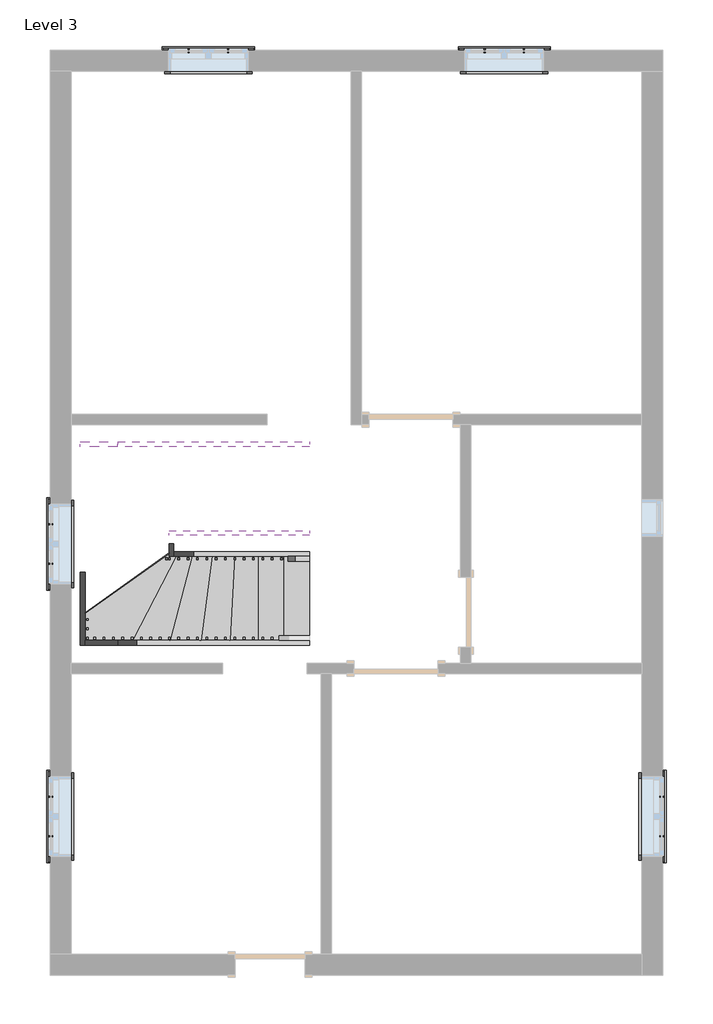
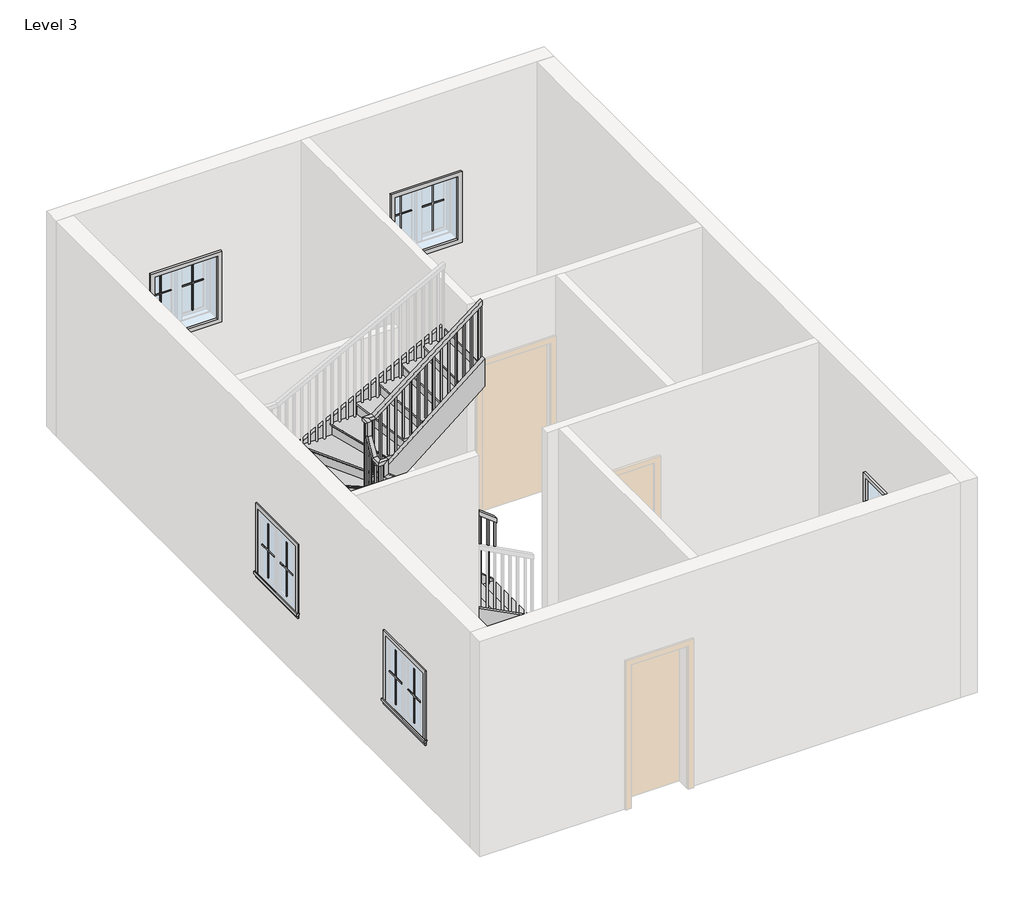
# One storey, part 2 of 2: 20 proxies, 8 members, 1 railing, 1 stair flight.
"""IFC4 building model written with IfcOpenShell, lengths in millimetres."""

from ifc_helpers import new_model, si_unit, frame, origin, place, context, project, spatial, polyline, outline, extrude, faceted_brep, transform, mapped, element, save
from components import muntin_pattern_2x2_muntin_pattern_2x2_b3fe6957, muntin_pattern_2x2_muntin_pattern_2x2_3e0ecaf2, trim_window_exterior_flat_with_sill_41619996, trim_window_interior_flat_picture_frame_51c85655, stair_flight_e257120f

model = new_model("IFC4")

# Units and contexts
model_context = context("Model", 3, world=origin())
ifc_project = project(units=[si_unit("LENGTHUNIT", "METRE", prefix="MILLI")], contexts=[model_context])

# Site, building, storey
site = spatial("IfcSite", under=ifc_project)
building = spatial("IfcBuilding", under=site)
storey = spatial("IfcBuildingStorey", under=building, Name="Level 3", Elevation=3200.4)

# Proxies
placement = place(None, origin())
muntin_pattern_2x2_muntin_pattern_2x2_shape = muntin_pattern_2x2_muntin_pattern_2x2_b3fe6957(model_context)
element("IfcBuildingElementProxy", 1, Name="Muntin Pattern_2x2 : Muntin Pattern_2x2", ObjectType="Muntin Pattern_2x2 : Muntin Pattern_2x2", at=placement, inside=storey, context=model_context, shape_type="MappedRepresentation", body=[
    mapped(muntin_pattern_2x2_muntin_pattern_2x2_shape, transform((-3096.8324167, 5150.2179147, 4184.65), x_axis=(1.0, 0.0, 0.0), y_axis=(0.0, 1.0, 0.0), z_axis=(0.0, 0.0, 1.0))),
])
element("IfcBuildingElementProxy", 2, Name="Muntin Pattern_2x2 : Muntin Pattern_2x2", ObjectType="Muntin Pattern_2x2 : Muntin Pattern_2x2", at=placement, inside=storey, context=model_context, shape_type="MappedRepresentation", body=[
    mapped(muntin_pattern_2x2_muntin_pattern_2x2_shape, transform((122.6175833, 5150.2179147, 4184.65), x_axis=(1.0, 0.0, 0.0), y_axis=(0.0, 1.0, 0.0), z_axis=(0.0, 0.0, 1.0))),
])
element("IfcBuildingElementProxy", 3, Name="Muntin Pattern_2x2 : Muntin Pattern_2x2", ObjectType="Muntin Pattern_2x2 : Muntin Pattern_2x2", at=placement, inside=storey, context=model_context, shape_type="MappedRepresentation", body=[
    mapped(muntin_pattern_2x2_muntin_pattern_2x2_shape, transform((2051.4300833, -2960.3195853, 4184.65), x_axis=(0.0, -1.0, 0.0), y_axis=(1.0, 0.0, 0.0), z_axis=(0.0, 0.0, 1.0))),
])
element("IfcBuildingElementProxy", 4, Name="Muntin Pattern_2x2 : Muntin Pattern_2x2", ObjectType="Muntin Pattern_2x2 : Muntin Pattern_2x2", at=placement, inside=storey, context=model_context, shape_type="MappedRepresentation", body=[
    mapped(muntin_pattern_2x2_muntin_pattern_2x2_shape, transform((-4597.0199167, -3388.9445853, 4184.65), x_axis=(0.0, 1.0, 0.0), y_axis=(-1.0, 0.0, 0.0), z_axis=(0.0, 0.0, 1.0))),
])
element("IfcBuildingElementProxy", 5, Name="Muntin Pattern_2x2 : Muntin Pattern_2x2", ObjectType="Muntin Pattern_2x2 : Muntin Pattern_2x2", at=placement, inside=storey, context=model_context, shape_type="MappedRepresentation", body=[
    mapped(muntin_pattern_2x2_muntin_pattern_2x2_shape, transform((-4597.0199167, -426.6695853, 4184.65), x_axis=(0.0, 1.0, 0.0), y_axis=(-1.0, 0.0, 0.0), z_axis=(0.0, 0.0, 1.0))),
])
muntin_pattern_2x2_muntin_pattern_2x2_2_shape = muntin_pattern_2x2_muntin_pattern_2x2_3e0ecaf2(model_context)
element("IfcBuildingElementProxy", 6, Name="Muntin Pattern_2x2 : Muntin Pattern_2x2", ObjectType="Muntin Pattern_2x2 : Muntin Pattern_2x2", at=placement, inside=storey, context=model_context, shape_type="MappedRepresentation", body=[
    mapped(muntin_pattern_2x2_muntin_pattern_2x2_2_shape, transform((-2668.2074167, 5150.2179147, 4184.65), x_axis=(-1.0, 0.0, 0.0), y_axis=(0.0, -1.0, 0.0), z_axis=(0.0, 0.0, 1.0))),
])
element("IfcBuildingElementProxy", 7, Name="Muntin Pattern_2x2 : Muntin Pattern_2x2", ObjectType="Muntin Pattern_2x2 : Muntin Pattern_2x2", at=placement, inside=storey, context=model_context, shape_type="MappedRepresentation", body=[
    mapped(muntin_pattern_2x2_muntin_pattern_2x2_2_shape, transform((551.2425833, 5150.2179147, 4184.65), x_axis=(-1.0, 0.0, 0.0), y_axis=(0.0, -1.0, 0.0), z_axis=(0.0, 0.0, 1.0))),
])
element("IfcBuildingElementProxy", 8, Name="Muntin Pattern_2x2 : Muntin Pattern_2x2", ObjectType="Muntin Pattern_2x2 : Muntin Pattern_2x2", at=placement, inside=storey, context=model_context, shape_type="MappedRepresentation", body=[
    mapped(muntin_pattern_2x2_muntin_pattern_2x2_2_shape, transform((2051.4300833, -3388.9445853, 4184.65), x_axis=(0.0, 1.0, 0.0), y_axis=(-1.0, 0.0, 0.0), z_axis=(0.0, 0.0, 1.0))),
])
element("IfcBuildingElementProxy", 9, Name="Muntin Pattern_2x2 : Muntin Pattern_2x2", ObjectType="Muntin Pattern_2x2 : Muntin Pattern_2x2", at=placement, inside=storey, context=model_context, shape_type="MappedRepresentation", body=[
    mapped(muntin_pattern_2x2_muntin_pattern_2x2_2_shape, transform((-4597.0199167, -2960.3195853, 4184.65), x_axis=(0.0, -1.0, 0.0), y_axis=(1.0, 0.0, 0.0), z_axis=(0.0, 0.0, 1.0))),
])
element("IfcBuildingElementProxy", 10, Name="Muntin Pattern_2x2 : Muntin Pattern_2x2", ObjectType="Muntin Pattern_2x2 : Muntin Pattern_2x2", at=placement, inside=storey, context=model_context, shape_type="MappedRepresentation", body=[
    mapped(muntin_pattern_2x2_muntin_pattern_2x2_2_shape, transform((-4597.0199167, 1.9554147, 4184.65), x_axis=(0.0, -1.0, 0.0), y_axis=(1.0, 0.0, 0.0), z_axis=(0.0, 0.0, 1.0))),
])
trim_window_exterior_flat_with_sill_shape = trim_window_exterior_flat_with_sill_41619996(model_context)
element("IfcBuildingElementProxy", 11, Name="Trim-Window-Exterior-Flat : with Sill", ObjectType="Trim-Window-Exterior-Flat : with Sill", at=placement, inside=storey, context=model_context, shape_type="MappedRepresentation", body=[
    mapped(trim_window_exterior_flat_with_sill_shape, transform((-2882.5199167, 5159.7429147, 5029.2), x_axis=(-1.0, 0.0, 0.0), y_axis=(0.0, 0.0, 1.0), z_axis=(0.0, 1.0, 0.0))),
])
element("IfcBuildingElementProxy", 12, Name="Trim-Window-Exterior-Flat : with Sill", ObjectType="Trim-Window-Exterior-Flat : with Sill", at=placement, inside=storey, context=model_context, shape_type="MappedRepresentation", body=[
    mapped(trim_window_exterior_flat_with_sill_shape, transform((336.9300833, 5159.7429147, 5029.2), x_axis=(-1.0, 0.0, 0.0), y_axis=(0.0, 0.0, 1.0), z_axis=(0.0, 1.0, 0.0))),
])
element("IfcBuildingElementProxy", 13, Name="Trim-Window-Exterior-Flat : with Sill", ObjectType="Trim-Window-Exterior-Flat : with Sill", at=placement, inside=storey, context=model_context, shape_type="MappedRepresentation", body=[
    mapped(trim_window_exterior_flat_with_sill_shape, transform((2060.9550833, -3174.6320853, 5029.2), x_axis=(0.0, 1.0, 0.0), y_axis=(0.0, 0.0, 1.0), z_axis=(1.0, 0.0, 0.0))),
])
element("IfcBuildingElementProxy", 14, Name="Trim-Window-Exterior-Flat : with Sill", ObjectType="Trim-Window-Exterior-Flat : with Sill", at=placement, inside=storey, context=model_context, shape_type="MappedRepresentation", body=[
    mapped(trim_window_exterior_flat_with_sill_shape, transform((-4606.5449167, -3174.6320853, 5029.2), x_axis=(0.0, -1.0, 0.0), y_axis=(0.0, 0.0, 1.0), z_axis=(-1.0, 0.0, 0.0))),
])
element("IfcBuildingElementProxy", 15, Name="Trim-Window-Exterior-Flat : with Sill", ObjectType="Trim-Window-Exterior-Flat : with Sill", at=placement, inside=storey, context=model_context, shape_type="MappedRepresentation", body=[
    mapped(trim_window_exterior_flat_with_sill_shape, transform((-4606.5449167, -212.3570853, 5029.2), x_axis=(0.0, -1.0, 0.0), y_axis=(0.0, 0.0, 1.0), z_axis=(-1.0, 0.0, 0.0))),
])
trim_window_interior_flat_picture_frame_shape = trim_window_interior_flat_picture_frame_51c85655(model_context)
element("IfcBuildingElementProxy", 16, Name="Trim-Window-Interior-Flat : Picture Frame", ObjectType="Trim-Window-Interior-Flat : Picture Frame", at=placement, inside=storey, context=model_context, shape_type="MappedRepresentation", body=[
    mapped(trim_window_interior_flat_picture_frame_shape, transform((-2882.5199167, 4931.1429147, 5029.2), x_axis=(1.0, 0.0, 0.0), y_axis=(0.0, 0.0, 1.0), z_axis=(0.0, -1.0, 0.0))),
])
element("IfcBuildingElementProxy", 17, Name="Trim-Window-Interior-Flat : Picture Frame", ObjectType="Trim-Window-Interior-Flat : Picture Frame", at=placement, inside=storey, context=model_context, shape_type="MappedRepresentation", body=[
    mapped(trim_window_interior_flat_picture_frame_shape, transform((336.9300833, 4931.1429147, 5029.2), x_axis=(1.0, 0.0, 0.0), y_axis=(0.0, 0.0, 1.0), z_axis=(0.0, -1.0, 0.0))),
])
element("IfcBuildingElementProxy", 18, Name="Trim-Window-Interior-Flat : Picture Frame", ObjectType="Trim-Window-Interior-Flat : Picture Frame", at=placement, inside=storey, context=model_context, shape_type="MappedRepresentation", body=[
    mapped(trim_window_interior_flat_picture_frame_shape, transform((1832.3550833, -3174.6320853, 5029.2), x_axis=(0.0, -1.0, 0.0), y_axis=(0.0, 0.0, 1.0), z_axis=(-1.0, 0.0, 0.0))),
])
element("IfcBuildingElementProxy", 19, Name="Trim-Window-Interior-Flat : Picture Frame", ObjectType="Trim-Window-Interior-Flat : Picture Frame", at=placement, inside=storey, context=model_context, shape_type="MappedRepresentation", body=[
    mapped(trim_window_interior_flat_picture_frame_shape, transform((-4377.9449167, -3174.6320853, 5029.2), x_axis=(0.0, 1.0, 0.0), y_axis=(0.0, 0.0, 1.0), z_axis=(1.0, 0.0, 0.0))),
])
element("IfcBuildingElementProxy", 20, Name="Trim-Window-Interior-Flat : Picture Frame", ObjectType="Trim-Window-Interior-Flat : Picture Frame", at=placement, inside=storey, context=model_context, shape_type="MappedRepresentation", body=[
    mapped(trim_window_interior_flat_picture_frame_shape, transform((-4377.9449167, -212.3570853, 5029.2), x_axis=(0.0, 1.0, 0.0), y_axis=(0.0, 0.0, 1.0), z_axis=(1.0, 0.0, 0.0))),
])

# Members
element("IfcMember", 21, ObjectType="Stringer - 2\" Width", at=placement, inside=storey, context=model_context, shape_type="SweptSolid", body=[
    extrude(outline(polyline([(3200.4, -1783.4132248), (3430.039954, -1783.4132248), (4505.7956453, -3870.8304165), (4162.900629, -3870.8304165), (3200.4, -2003.1755424), (3200.4, -1783.4132248)])), frame((0.0, -1310.9070853, 0.0), z_axis=(0.0, 1.0, 0.0), x_axis=(0.0, 0.0, 1.0)), (0.0, 0.0, 1.0), 50.8),
])
element("IfcMember", 22, ObjectType="Stringer - 2\" Width", at=placement, inside=storey, context=model_context, shape_type="SweptSolid", body=[
    extrude(outline(polyline([(-3870.8304165, -1260.1070853), (-3870.8304165, -1310.9070853), (-4225.5449167, -1310.9070853), (-4225.5449167, -1260.1070853), (-3870.8304165, -1260.1070853)])), frame((0.0, 0.0, 4162.900629), z_axis=(0.0, 0.0, 1.0), x_axis=(1.0, 0.0, 0.0)), (0.0, 0.0, 1.0), 342.8950162),
])
element("IfcMember", 23, ObjectType="Stringer - 2\" Width", at=placement, inside=storey, context=model_context, shape_type="SweptSolid", body=[
    extrude(outline(polyline([(-1310.9070853, 4200.9956453), (-1310.9070853, 4489.4952212), (811.1127974, 5170.3972697), (848.0929147, 5170.3972697), (848.0929147, 4839.3682298), (-1141.3846024, 4200.9956453), (-1310.9070853, 4200.9956453)])), frame((-4276.3449167, 0.0, 0.0), z_axis=(1.0, 0.0, 0.0), x_axis=(0.0, 1.0, 0.0)), (0.0, 0.0, 1.0), 50.8),
])
element("IfcMember", 24, ObjectType="Stringer - 2\" Width", at=placement, inside=storey, context=model_context, shape_type="SweptSolid", body=[
    extrude(outline(polyline([(-4276.3449167, 848.0929147), (-4276.3449167, 898.8929147), (-3870.8304165, 898.8929147), (-3870.8304165, 848.0929147), (-4276.3449167, 848.0929147)])), frame((0.0, 0.0, 4850.2904473), z_axis=(0.0, 0.0, 1.0), x_axis=(1.0, 0.0, 0.0)), (0.0, 0.0, 1.0), 320.1068224),
])
element("IfcMember", 25, ObjectType="Stringer - 2\" Width", at=placement, inside=storey, context=model_context, shape_type="SweptSolid", body=[
    extrude(outline(polyline([(5170.3972697, -3870.8304165), (4850.2904473, -3870.8304165), (5926.0461385, -1783.4132248), (6246.1529609, -1783.4132248), (5170.3972697, -3870.8304165)])), frame((0.0, 848.0929147, 0.0), z_axis=(0.0, 1.0, 0.0), x_axis=(0.0, 0.0, 1.0)), (0.0, 0.0, 1.0), 50.8),
])
element("IfcMember", 26, ObjectType="Stringer - 2\" Width", at=placement, inside=storey, context=model_context, shape_type="SweptSolid", body=[
    extrude(outline(polyline([(3200.4, -1783.4132248), (3376.5764461, -1783.4132248), (4580.818648, -3260.3449167), (4187.5410923, -3260.3449167), (3200.4, -2049.6748694), (3200.4, -1783.4132248)])), frame((0.0, -345.7070853, 0.0), z_axis=(0.0, 1.0, 0.0), x_axis=(0.0, 0.0, 1.0)), (0.0, 0.0, 1.0), 50.8),
])
element("IfcMember", 27, ObjectType="Stringer - 2\" Width", at=placement, inside=storey, context=model_context, shape_type="SweptSolid", body=[
    extrude(outline(polyline([(-345.7070853, 4228.9617647), (-345.7070853, 4773.6682978), (-139.0699679, 5126.5409689), (-117.1070853, 5126.5409689), (-117.1070853, 4560.865107), (-311.464868, 4228.9617647), (-345.7070853, 4228.9617647)])), frame((-3311.1449167, 0.0, 0.0), z_axis=(1.0, 0.0, 0.0), x_axis=(0.0, 1.0, 0.0)), (0.0, 0.0, 1.0), 50.8),
])
element("IfcMember", 28, ObjectType="Stringer - 2\" Width", at=placement, inside=storey, context=model_context, shape_type="SweptSolid", body=[
    extrude(outline(polyline([(5126.5409689, -3311.1449167), (4733.2634131, -3311.1449167), (5978.9262875, -1783.4132248), (6372.2038432, -1783.4132248), (5126.5409689, -3311.1449167)])), frame((0.0, -117.1070853, 0.0), z_axis=(0.0, 1.0, 0.0), x_axis=(0.0, 0.0, 1.0)), (0.0, 0.0, 1.0), 50.8),
])

# Railing
element("IfcRailing", 29, ObjectType="Handrail - Rectangular", at=placement, inside=storey, context=model_context, shape_type="SolidModel", body=[
    faceted_brep([(-1783.4132248, -396.5070853, 4284.1333333), (-1783.4132248, -396.5070853, 4219.8000346), (-1783.4132248, -345.7070853, 4219.8000346), (-1783.4132248, -345.7070853, 4284.1333333), (-3234.9449167, -396.5070853, 5412.0191036), (-3285.7449167, -396.5070853, 5387.1590024), (-3285.7449167, -345.7070853, 5387.1590024), (-3234.9449167, -345.7070853, 5412.0191036), (-3234.9449167, -396.5070853, 5615.0281882), (-3285.7449167, -396.5070853, 5564.2281882), (-3285.7449167, -345.7070853, 5564.2281882), (-3234.9449167, -345.7070853, 5615.0281882), (-3361.9449167, -396.5070853, 5615.0281882), (-3361.9449167, -396.5070853, 5564.2281882), (-3311.1449167, -345.7070853, 5564.2281882), (-3311.1449167, -345.7070853, 5615.0281882), (-3361.9449167, -269.5070853, 5615.0281882), (-3361.9449167, -240.3857515, 5564.2281882), (-3311.1449167, -240.3857515, 5564.2281882), (-3311.1449167, -269.5070853, 5615.0281882), (-3361.9449167, -142.5070853, 5831.9051451), (-3361.9449167, -91.7070853, 5818.1256424), (-3311.1449167, -91.7070853, 5818.1256424), (-3311.1449167, -142.5070853, 5831.9051451), (-3361.9449167, -142.5070853, 6034.9142297), (-3361.9449167, -91.7070853, 5984.1142297), (-3311.1449167, -91.7070853, 5984.1142297), (-3311.1449167, -142.5070853, 6034.9142297), (-3361.9449167, -15.5070853, 6034.9142297), (-3361.9449167, -15.5070853, 5984.1142297), (-3311.1449167, -66.3070853, 5984.1142297), (-3311.1449167, -66.3070853, 6034.9142297), (-3234.9449167, -15.5070853, 6034.9142297), (-3217.5282487, -15.5070853, 5984.1142297), (-3217.5282487, -66.3070853, 5984.1142297), (-3234.9449167, -66.3070853, 6034.9142297), (-1783.4132248, -15.5070853, 7162.8), (-1783.4132248, -66.3070853, 7162.8), (-1783.4132248, -66.3070853, 7098.4667013), (-1783.4132248, -15.5070853, 7098.4667013)], [[[0, 1, 2, 3]], [[1, 0, 4, 5]], [[2, 1, 5, 6]], [[3, 2, 6, 7]], [[0, 3, 7, 4]], [[5, 4, 8, 9]], [[6, 5, 9, 10]], [[7, 6, 10, 11]], [[4, 7, 11, 8]], [[9, 8, 12, 13]], [[10, 9, 13, 14]], [[11, 10, 14, 15]], [[8, 11, 15, 12]], [[13, 12, 16, 17]], [[14, 13, 17, 18]], [[15, 14, 18, 19]], [[12, 15, 19, 16]], [[17, 16, 20, 21]], [[18, 17, 21, 22]], [[19, 18, 22, 23]], [[16, 19, 23, 20]], [[21, 20, 24, 25]], [[22, 21, 25, 26]], [[23, 22, 26, 27]], [[20, 23, 27, 24]], [[25, 24, 28, 29]], [[26, 25, 29, 30]], [[27, 26, 30, 31]], [[24, 27, 31, 28]], [[29, 28, 32, 33]], [[30, 29, 33, 34]], [[31, 30, 34, 35]], [[28, 31, 35, 32]], [[36, 37, 38, 39]], [[33, 32, 36, 39]], [[34, 33, 39, 38]], [[35, 34, 38, 37]], [[32, 35, 37, 36]]]),
    extrude(outline(polyline([(7083.2316852, -1803.0199167), (7068.4292361, -1822.0699167), (6079.0666667, -1822.0699167), (6079.0666667, -1803.0199167), (7083.2316852, -1803.0199167)])), frame((0.0, -50.4320853, 0.0), z_axis=(0.0, 1.0, 0.0), x_axis=(0.0, 0.0, 1.0)), (0.0, 0.0, 1.0), 19.05),
    extrude(outline(polyline([(7004.2852902, -1904.6199167), (6989.4828411, -1923.6699167), (6079.0666667, -1923.6699167), (6079.0666667, -1904.6199167), (7004.2852902, -1904.6199167)])), frame((0.0, -50.4320853, 0.0), z_axis=(0.0, 1.0, 0.0), x_axis=(0.0, 0.0, 1.0)), (0.0, 0.0, 1.0), 19.05),
    extrude(outline(polyline([(6925.3388952, -2006.2199167), (6910.5364462, -2025.2699167), (6079.0666667, -2025.2699167), (6079.0666667, -2006.2199167), (6925.3388952, -2006.2199167)])), frame((0.0, -50.4320853, 0.0), z_axis=(0.0, 1.0, 0.0), x_axis=(0.0, 0.0, 1.0)), (0.0, 0.0, 1.0), 19.05),
    extrude(outline(polyline([(6846.3925003, -2107.8199167), (6831.5900512, -2126.8699167), (5909.7333333, -2126.8699167), (5909.7333333, -2107.8199167), (6846.3925003, -2107.8199167)])), frame((0.0, -50.4320853, 0.0), z_axis=(0.0, 1.0, 0.0), x_axis=(0.0, 0.0, 1.0)), (0.0, 0.0, 1.0), 19.05),
    extrude(outline(polyline([(6767.4461053, -2209.4199167), (6752.6436562, -2228.4699167), (5909.7333333, -2228.4699167), (5909.7333333, -2209.4199167), (6767.4461053, -2209.4199167)])), frame((0.0, -50.4320853, 0.0), z_axis=(0.0, 1.0, 0.0), x_axis=(0.0, 0.0, 1.0)), (0.0, 0.0, 1.0), 19.05),
    extrude(outline(polyline([(6688.4997103, -2311.0199167), (6673.6972613, -2330.0699167), (5909.7333333, -2330.0699167), (5909.7333333, -2311.0199167), (6688.4997103, -2311.0199167)])), frame((0.0, -50.4320853, 0.0), z_axis=(0.0, 1.0, 0.0), x_axis=(0.0, 0.0, 1.0)), (0.0, 0.0, 1.0), 19.05),
    extrude(outline(polyline([(6609.5533154, -2412.6199167), (6594.7508663, -2431.6699167), (5740.4, -2431.6699167), (5740.4, -2412.6199167), (6609.5533154, -2412.6199167)])), frame((0.0, -50.4320853, 0.0), z_axis=(0.0, 1.0, 0.0), x_axis=(0.0, 0.0, 1.0)), (0.0, 0.0, 1.0), 19.05),
    extrude(outline(polyline([(6530.6069204, -2514.2199167), (6515.8044713, -2533.2699167), (5740.4, -2533.2699167), (5740.4, -2514.2199167), (6530.6069204, -2514.2199167)])), frame((0.0, -50.4320853, 0.0), z_axis=(0.0, 1.0, 0.0), x_axis=(0.0, 0.0, 1.0)), (0.0, 0.0, 1.0), 19.05),
    extrude(outline(polyline([(6451.6605254, -2615.8199167), (6436.8580764, -2634.8699167), (5571.0666667, -2634.8699167), (5571.0666667, -2615.8199167), (6451.6605254, -2615.8199167)])), frame((0.0, -50.4320853, 0.0), z_axis=(0.0, 1.0, 0.0), x_axis=(0.0, 0.0, 1.0)), (0.0, 0.0, 1.0), 19.05),
    extrude(outline(polyline([(6372.7141304, -2717.4199167), (6357.9116814, -2736.4699167), (5571.0666667, -2736.4699167), (5571.0666667, -2717.4199167), (6372.7141304, -2717.4199167)])), frame((0.0, -50.4320853, 0.0), z_axis=(0.0, 1.0, 0.0), x_axis=(0.0, 0.0, 1.0)), (0.0, 0.0, 1.0), 19.05),
    extrude(outline(polyline([(6293.7677355, -2819.0199167), (6278.9652864, -2838.0699167), (5571.0666667, -2838.0699167), (5571.0666667, -2819.0199167), (6293.7677355, -2819.0199167)])), frame((0.0, -50.4320853, 0.0), z_axis=(0.0, 1.0, 0.0), x_axis=(0.0, 0.0, 1.0)), (0.0, 0.0, 1.0), 19.05),
    extrude(outline(polyline([(6214.8213405, -2920.6199167), (6200.0188914, -2939.6699167), (5401.7333333, -2939.6699167), (5401.7333333, -2920.6199167), (6214.8213405, -2920.6199167)])), frame((0.0, -50.4320853, 0.0), z_axis=(0.0, 1.0, 0.0), x_axis=(0.0, 0.0, 1.0)), (0.0, 0.0, 1.0), 19.05),
    extrude(outline(polyline([(6135.8749455, -3022.2199167), (6121.0724965, -3041.2699167), (5401.7333333, -3041.2699167), (5401.7333333, -3022.2199167), (6135.8749455, -3022.2199167)])), frame((0.0, -50.4320853, 0.0), z_axis=(0.0, 1.0, 0.0), x_axis=(0.0, 0.0, 1.0)), (0.0, 0.0, 1.0), 19.05),
    extrude(outline(polyline([(6056.9285506, -3123.8199167), (6042.1261015, -3142.8699167), (5232.4, -3142.8699167), (5232.4, -3123.8199167), (6056.9285506, -3123.8199167)])), frame((0.0, -50.4320853, 0.0), z_axis=(0.0, 1.0, 0.0), x_axis=(0.0, 0.0, 1.0)), (0.0, 0.0, 1.0), 19.05),
    extrude(outline(polyline([(5977.9821556, -3225.4199167), (5963.1797065, -3244.4699167), (5232.4, -3244.4699167), (5232.4, -3225.4199167), (5977.9821556, -3225.4199167)])), frame((0.0, -50.4320853, 0.0), z_axis=(0.0, 1.0, 0.0), x_axis=(0.0, 0.0, 1.0)), (0.0, 0.0, 1.0), 19.05),
    extrude(outline(polyline([(-3327.0199167, -75.8320853), (-3346.0699167, -75.8320853), (-3346.0699167, -56.7820853), (-3327.0199167, -56.7820853), (-3327.0199167, -75.8320853)])), frame((0.0, 0.0, 4893.7333333), z_axis=(0.0, 0.0, 1.0), x_axis=(1.0, 0.0, 0.0)), (0.0, 0.0, 1.0), 1090.3808964),
    extrude(outline(polyline([(-177.4320853, 5671.7336964), (-158.3820853, 5704.26524), (-158.3820853, 4724.4), (-177.4320853, 4724.4), (-177.4320853, 5671.7336964)])), frame((-3346.0699167, 0.0, 0.0), z_axis=(1.0, 0.0, 0.0), x_axis=(0.0, 1.0, 0.0)), (0.0, 0.0, 1.0), 19.05),
    extrude(outline(polyline([(-279.0320853, 5498.2321309), (-259.9820853, 5530.7636744), (-259.9820853, 4555.0666667), (-279.0320853, 4555.0666667), (-279.0320853, 5498.2321309)])), frame((-3346.0699167, 0.0, 0.0), z_axis=(1.0, 0.0, 0.0), x_axis=(0.0, 1.0, 0.0)), (0.0, 0.0, 1.0), 19.05),
    extrude(outline(polyline([(-3297.8882248, -361.5820853), (-3297.8882248, -380.6320853), (-3316.9382248, -380.6320853), (-3316.9382248, -361.5820853), (-3297.8882248, -361.5820853)])), frame((0.0, 0.0, 4385.7333333), z_axis=(0.0, 0.0, 1.0), x_axis=(1.0, 0.0, 0.0)), (0.0, 0.0, 1.0), 1178.4948549),
    extrude(outline(polyline([(5317.6483397, -3196.2882248), (5332.4507888, -3215.3382248), (4216.4, -3215.3382248), (4216.4, -3196.2882248), (5317.6483397, -3196.2882248)])), frame((0.0, -380.6320853, 0.0), z_axis=(0.0, 1.0, 0.0), x_axis=(0.0, 0.0, 1.0)), (0.0, 0.0, 1.0), 19.05),
    extrude(outline(polyline([(5238.7019447, -3094.6882248), (5253.5043938, -3113.7382248), (4216.4, -3113.7382248), (4216.4, -3094.6882248), (5238.7019447, -3094.6882248)])), frame((0.0, -380.6320853, 0.0), z_axis=(0.0, 1.0, 0.0), x_axis=(0.0, 0.0, 1.0)), (0.0, 0.0, 1.0), 19.05),
    extrude(outline(polyline([(5159.7555498, -2993.0882248), (5174.5579988, -3012.1382248), (4047.0666667, -3012.1382248), (4047.0666667, -2993.0882248), (5159.7555498, -2993.0882248)])), frame((0.0, -380.6320853, 0.0), z_axis=(0.0, 1.0, 0.0), x_axis=(0.0, 0.0, 1.0)), (0.0, 0.0, 1.0), 19.05),
    extrude(outline(polyline([(5080.8091548, -2891.4882248), (5095.6116039, -2910.5382248), (4047.0666667, -2910.5382248), (4047.0666667, -2891.4882248), (5080.8091548, -2891.4882248)])), frame((0.0, -380.6320853, 0.0), z_axis=(0.0, 1.0, 0.0), x_axis=(0.0, 0.0, 1.0)), (0.0, 0.0, 1.0), 19.05),
    extrude(outline(polyline([(5001.8627598, -2789.8882248), (5016.6652089, -2808.9382248), (3877.7333333, -2808.9382248), (3877.7333333, -2789.8882248), (5001.8627598, -2789.8882248)])), frame((0.0, -380.6320853, 0.0), z_axis=(0.0, 1.0, 0.0), x_axis=(0.0, 0.0, 1.0)), (0.0, 0.0, 1.0), 19.05),
    extrude(outline(polyline([(4922.9163649, -2688.2882248), (4937.7188139, -2707.3382248), (3877.7333333, -2707.3382248), (3877.7333333, -2688.2882248), (4922.9163649, -2688.2882248)])), frame((0.0, -380.6320853, 0.0), z_axis=(0.0, 1.0, 0.0), x_axis=(0.0, 0.0, 1.0)), (0.0, 0.0, 1.0), 19.05),
    extrude(outline(polyline([(4843.9699699, -2586.6882248), (4858.7724189, -2605.7382248), (3708.4, -2605.7382248), (3708.4, -2586.6882248), (4843.9699699, -2586.6882248)])), frame((0.0, -380.6320853, 0.0), z_axis=(0.0, 1.0, 0.0), x_axis=(0.0, 0.0, 1.0)), (0.0, 0.0, 1.0), 19.05),
    extrude(outline(polyline([(4765.0235749, -2485.0882248), (4779.826024, -2504.1382248), (3708.4, -2504.1382248), (3708.4, -2485.0882248), (4765.0235749, -2485.0882248)])), frame((0.0, -380.6320853, 0.0), z_axis=(0.0, 1.0, 0.0), x_axis=(0.0, 0.0, 1.0)), (0.0, 0.0, 1.0), 19.05),
    extrude(outline(polyline([(4686.0771799, -2383.4882248), (4700.879629, -2402.5382248), (3708.4, -2402.5382248), (3708.4, -2383.4882248), (4686.0771799, -2383.4882248)])), frame((0.0, -380.6320853, 0.0), z_axis=(0.0, 1.0, 0.0), x_axis=(0.0, 0.0, 1.0)), (0.0, 0.0, 1.0), 19.05),
    extrude(outline(polyline([(4607.130785, -2281.8882248), (4621.933234, -2300.9382248), (3539.0666667, -2300.9382248), (3539.0666667, -2281.8882248), (4607.130785, -2281.8882248)])), frame((0.0, -380.6320853, 0.0), z_axis=(0.0, 1.0, 0.0), x_axis=(0.0, 0.0, 1.0)), (0.0, 0.0, 1.0), 19.05),
    extrude(outline(polyline([(4528.18439, -2180.2882248), (4542.9868391, -2199.3382248), (3539.0666667, -2199.3382248), (3539.0666667, -2180.2882248), (4528.18439, -2180.2882248)])), frame((0.0, -380.6320853, 0.0), z_axis=(0.0, 1.0, 0.0), x_axis=(0.0, 0.0, 1.0)), (0.0, 0.0, 1.0), 19.05),
    extrude(outline(polyline([(4449.237995, -2078.6882248), (4464.0404441, -2097.7382248), (3539.0666667, -2097.7382248), (3539.0666667, -2078.6882248), (4449.237995, -2078.6882248)])), frame((0.0, -380.6320853, 0.0), z_axis=(0.0, 1.0, 0.0), x_axis=(0.0, 0.0, 1.0)), (0.0, 0.0, 1.0), 19.05),
    extrude(outline(polyline([(4370.2916001, -1977.0882248), (4385.0940491, -1996.1382248), (3369.7333333, -1996.1382248), (3369.7333333, -1977.0882248), (4370.2916001, -1977.0882248)])), frame((0.0, -380.6320853, 0.0), z_axis=(0.0, 1.0, 0.0), x_axis=(0.0, 0.0, 1.0)), (0.0, 0.0, 1.0), 19.05),
    extrude(outline(polyline([(4291.3452051, -1875.4882248), (4306.1476541, -1894.5382248), (3369.7333333, -1894.5382248), (3369.7333333, -1875.4882248), (4291.3452051, -1875.4882248)])), frame((0.0, -380.6320853, 0.0), z_axis=(0.0, 1.0, 0.0), x_axis=(0.0, 0.0, 1.0)), (0.0, 0.0, 1.0), 19.05),
    extrude(outline(polyline([(-3327.0199167, -50.4320853), (-3346.0699167, -50.4320853), (-3346.0699167, -31.3820853), (-3327.0199167, -31.3820853), (-3327.0199167, -50.4320853)])), frame((0.0, 0.0, 5063.0666667), z_axis=(0.0, 0.0, 1.0), x_axis=(1.0, 0.0, 0.0)), (0.0, 0.0, 1.0), 921.0475631),
    extrude(outline(polyline([(-3327.0199167, -361.5820853), (-3327.0199167, -380.6320853), (-3346.0699167, -380.6320853), (-3346.0699167, -361.5820853), (-3327.0199167, -361.5820853)])), frame((0.0, 0.0, 4385.7333333), z_axis=(0.0, 0.0, 1.0), x_axis=(1.0, 0.0, 0.0)), (0.0, 0.0, 1.0), 1178.4948549),
    extrude(outline(polyline([(7098.4667013, -1783.4132248), (7083.6642523, -1802.4632248), (6079.0666667, -1802.4632248), (6079.0666667, -1783.4132248), (7098.4667013, -1783.4132248)])), frame((0.0, -50.4320853, 0.0), z_axis=(0.0, 1.0, 0.0), x_axis=(0.0, 0.0, 1.0)), (0.0, 0.0, 1.0), 19.05),
    extrude(outline(polyline([(4219.8000346, -1783.4132248), (4234.6024837, -1802.4632248), (3369.7333333, -1802.4632248), (3369.7333333, -1783.4132248), (4219.8000346, -1783.4132248)])), frame((0.0, -380.6320853, 0.0), z_axis=(0.0, 1.0, 0.0), x_axis=(0.0, 0.0, 1.0)), (0.0, 0.0, 1.0), 19.05),
])

# Stair flight
stair_flight_shape = stair_flight_e257120f(model_context)
element("IfcStairFlight", 30, ObjectType="2\" Tread 1\" Nosing 1/4\" Riser", at=placement, inside=storey, context=model_context, shape_type="MappedRepresentation", body=[
    mapped(stair_flight_shape, transform((0.0, 0.0, 0.0), x_axis=(1.0, 0.0, 0.0), y_axis=(0.0, 1.0, 0.0), z_axis=(0.0, 0.0, 1.0))),
])

save(model, "model.ifc")

# Revit data of these elements
# Type "Muntin Pattern_2x2 : Muntin Pattern_2x2"
#   Width [instance default] = 4' - 0"
#   Thickness = 0' - 0 1/2"
#   Height [instance default] = 4' - 0"
#   Distance = 0' - 0 3/4"
#   Interior Material [instance default] = none
#   Exterior Material [instance default] = none
#   Default Elevation = 0
# Type "Trim-Window-Exterior-Flat : with Sill"
#   Trim Width = 0' - 2 1/4"
#   Trim Thickness_Picture Frame = 0' - 1 1/4"
#   Trim Thickness_with Sill = 0' - 0 3/4"
#   Sill Thickness = 0' - 1 1/4"
#   Opening Width [instance default] = 2' - 0"
#   Opening Height [instance default] = 3' - 0"
#   Default Elevation = 4' - 0"
#   Sill = yes
#   Picture Frame = no
#   Trim Material [instance default] = none
# Type "Trim-Window-Interior-Flat : Picture Frame"
#   Trim Thickness_Picture Frame = 0' - 1 1/4"
#   Trim Width = 0' - 2 1/4"
#   Trim Thickness_with Sill = 0' - 0 3/4"
#   Sill Thickness = 0' - 1 1/4"
#   Opening Width [instance default] = 2' - 0"
#   Opening Height [instance default] = 3' - 0"
#   Default Elevation = 4' - 0"
#   Sill = no
#   Picture Frame = yes
#   Trim Material [instance default] = none
# Type "Handrail - Rectangular"
#   Assembly Code = "C2010400"
#   built-in parameter 1008612 = 0.0416667 (stored number, unit not read)
#   built-in parameter 1008611 = 0.0416667 (stored number, unit not read)
#   built-in parameter 1008609 = 0.333333 (stored number, unit not read)
#   built-in parameter 1008604 = 0.166667 (stored number, unit not read)
#   built-in parameter 1008603 = 0.166667 (stored number, unit not read)
#   Railing Height = 3' - 0"
#   built-in parameter 1008630 = 2
#   built-in parameter 1008610 = 2
#   built-in parameter 1008618 = Baluster - Square : 3/4"
# Elements 1, 2, 3, 4, 5, 6, 7, 8, 9, 10 (IfcBuildingElementProxy, "Muntin Pattern_2x2 : Muntin Pattern_2x2")
#   Width = 0' - 11 5/8"
#   Height = 2' - 6 1/2"
#   Interior Material = Wood - Stained
#   Exterior Material = Clad - White
#   Phase Created = New Construction
#   Materials on its faces: "Clad - White", "Wood - Stained"
# Elements 11, 12, 13, 14, 15 (IfcBuildingElementProxy, "Trim-Window-Exterior-Flat : with Sill")
#   Opening Width = 2' - 10"
#   Opening Height = 3' - 0"
#   Trim Material = Clad - White
#   Phase Created = New Construction
#   Materials on its faces: "Clad - White"
# Elements 16, 17, 18, 19, 20 (IfcBuildingElementProxy, "Trim-Window-Interior-Flat : Picture Frame")
#   Opening Width = 2' - 10"
#   Opening Height = 3' - 0"
#   Trim Material = Wood - Stained
#   Phase Created = New Construction
#   Materials on its faces: "Wood - Stained"
# Elements 21, 22, 23, 24, 25, 26, 27, 28 (IfcMember, "Stringer - 2\" Width")
#   Phase Created = New Construction
# Element 29 (IfcRailing, "Handrail - Rectangular")
#   Phase Created = New Construction
# Element 30 (IfcStairFlight, "2\" Tread 1\" Nosing 1/4\" Riser")
#   Phase Created = New Construction
# Materials
#   "Clad - White": class "Wood", colour RGB 242 242 238, transparency 0, Cost = 0
#   "Wood - Stained": class "Wood", colour RGB 224 178 126, transparency 0, Cost = 0
